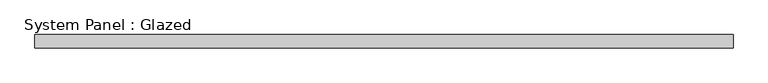
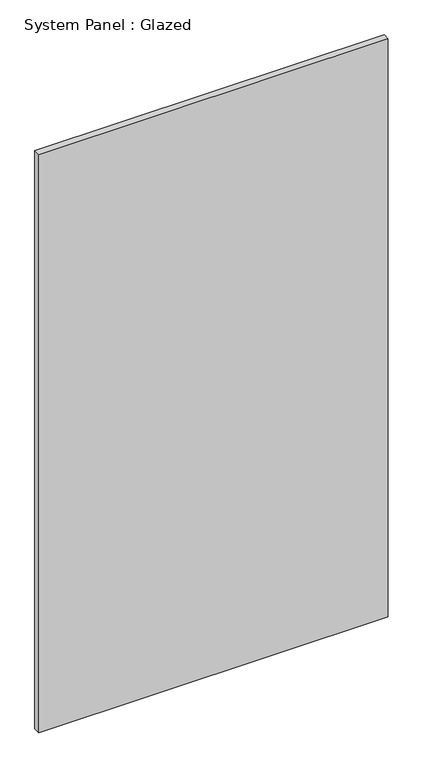
"""IFC4 building model written with IfcOpenShell, lengths in millimetres: plate geometry, System Panel : Glazed."""

from ifc_helpers import new_model, si_unit, origin, origin_with_axes, place, context, project, spatial, polyline, outline, extrude, source, transform, mapped, element, save


def system_panel_glazed_bd4b6abd(model_context):
    return source(origin(), model_context, "Body", "SweptSolid", [
        extrude(outline(polyline([(669.9250001, 19.05), (-669.9250001, 19.05), (-669.9250001, 44.45), (669.9250001, 44.45), (669.9250001, 19.05)])), origin_with_axes(), (0.0, 0.0, 1.0), 2343.15),
    ])


if __name__ == "__main__":
    model = new_model("IFC4")
    model_context = context("Model", 3, world=origin())
    ifc_project = project(units=[si_unit("LENGTHUNIT", "METRE", prefix="MILLI")], contexts=[model_context])
    site = spatial("IfcSite", under=ifc_project)
    building = spatial("IfcBuilding", under=site)
    placement = place(None, origin())
    system_panel_glazed_shape = system_panel_glazed_bd4b6abd(model_context)
    element("IfcPlate", 1, ObjectType="System Panel : Glazed", at=placement, inside=building, context=model_context, shape_type="MappedRepresentation", body=[
        mapped(system_panel_glazed_shape, transform((0.0, 0.0, 0.0), x_axis=(1.0, 0.0, 0.0), y_axis=(0.0, 1.0, 0.0), z_axis=(0.0, 0.0, 1.0))),
    ])
    save(model, "model.ifc")

# Revit data of these elements
# Type "System Panel : Glazed"
#   Construction Type Id = "GSP4R"
#   Analytic Construction = "1/8 in Pilkington single glazing"
#   Visual Light Transmittance = 0.9
#   Solar Heat Gain Coefficient = 0.86
#   Heat Transfer Coefficient (U) = 1.18115 BTU/(h·ft²·°F)
#   Define Thermal Properties by = 1
# Element 1 (IfcPlate, "System Panel : Glazed")
#   Materials on its faces: "Glass"
# Materials
#   "Glass": class "Glass", colour RGB 0 128 192, transparency 0.75, Description = "Soda Lime Glass", Cost = 0
